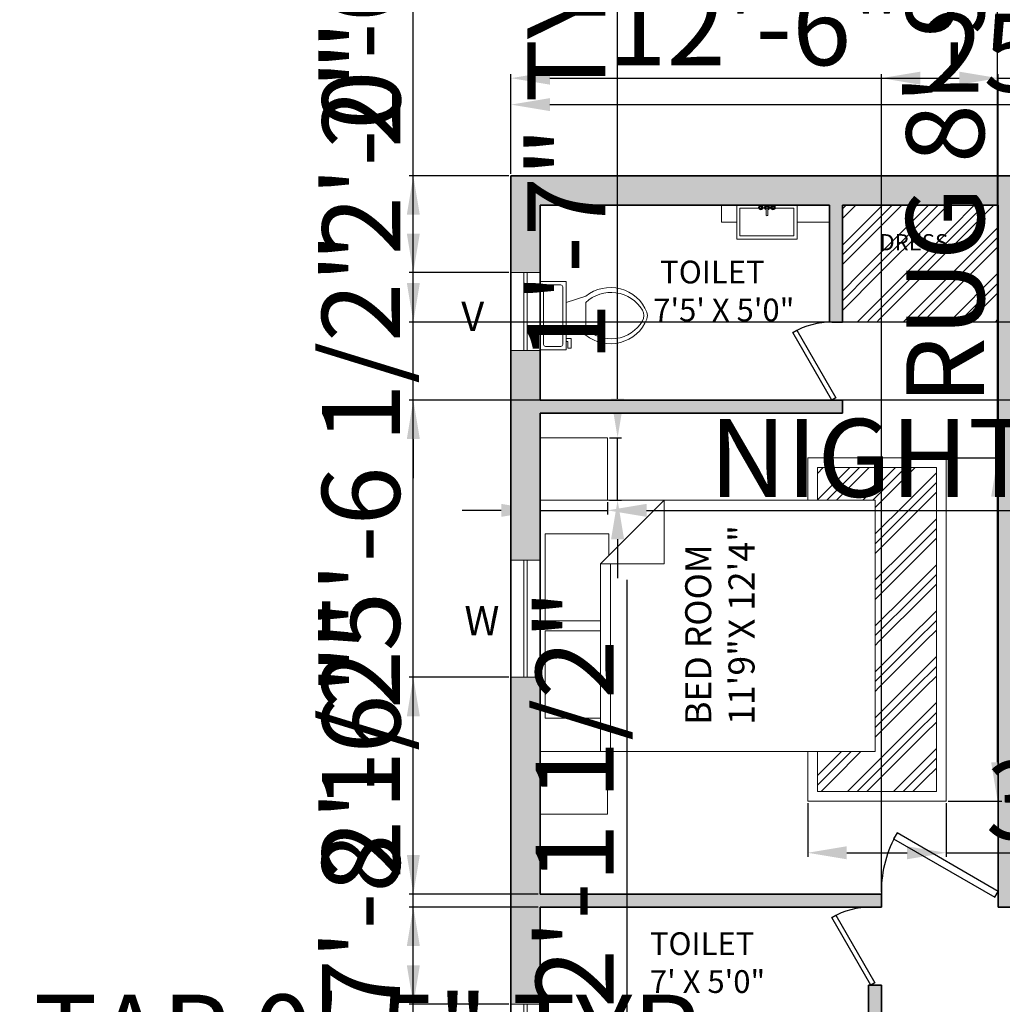
# Model space of a CAD drawing. Units: inches. Extents: x 830 to 1639, y 2591 to 3595.
# Tile 3 of 7: x 830 to 1133, y 2957 to 3260. Entities that reach past the tile are written whole.
import ezdxf

# ---------------------------------------------------------------- set-up
doc = ezdxf.new("R2010")
doc.units = ezdxf.units.IN
doc.layers.get('0').update_dxf_attribs({"color": 250})
for name, color, linetype, lineweight in [('A-ANNO-DIMS', 2, 'Continuous', 18), ('A-ANNO-TEXT', 7, 'Continuous', 18), ('A-AREA-IDEN', 7, 'Continuous', 25), ('A-DOOR', 3, 'Continuous', 25), ('A-FLOR-CASE', 8, 'Continuous', 18), ('A-FLOR-FIXT', 8, 'Continuous', 18), ('A-FLOR-PATT', 252, 'Continuous', 13), ('A-FURN', 8, 'Continuous', 18), ('A-GLAZ', 4, 'Continuous', 18), ('A-WALL', 7, 'Continuous', 35), ('A-WALL-PATT', 5, 'Continuous', 13), ('C-PROP', 7, 'Continuous', 35)]:
    doc.layers.add(name, color=color, linetype=linetype, lineweight=lineweight)
doc.styles.get("Standard").update_dxf_attribs({"font": 'arial.ttf'})
doc.dimstyles.new('ISO-25', dxfattribs={"dimtxt": 24, "dimasz": 12, "dimexe": 1.25, "dimexo": 0.625, "dimtad": 1, "dimdec": 0, "dimlunit": 3, "dimtxsty": 'Standard', "dimcen": 2.5, "dimadec": 0, "dimazin": 0, "dimtfac": 1, "dimtdec": 0, "dimtmove": 0, "dimatfit": 3, "dimfxl": 1, "dimarcsym": 0})

# ---------------------------------------------------------------- blocks, each defined once
blk = doc.blocks.new('Faucet - Bathroom top')
for p, q in [((-4.107, 0.125), (-4.375, 0.125)), ((-3.75, 0.4788), (-3.75, 0.75)), ((-3.5, 0.482), (-3.5, 0.75)), ((-3.1461, 0.125), (-2.875, 0.125)), ((3.143, 0.125), (2.875, 0.125)), ((3.5, 0.4788), (3.5, 0.75)), ((3.75, 0.482), (3.75, 0.75)), ((4.1039, 0.125), (4.375, 0.125)), ((-4.1039, -0.125), (-4.375, -0.125)), ((-3.75, -0.4821), (-3.75, -0.75)), ((-3.5, -0.4789), (-3.5, -0.75)), ((-3.143, -0.125), (-2.875, -0.125)), ((-0.5, -0.8639), (-0.5, -4.5)), ((0.5, -4.5), (0.5, -0.8631)), ((3.1461, -0.125), (2.875, -0.125)), ((3.5, -0.4821), (3.5, -0.75)), ((3.75, -0.4789), (3.75, -0.75)), ((4.107, -0.125), (4.375, -0.125))]:
    blk.add_line(p, q)
for centre, radius in [((-3.625, 0), 1.375), ((-4.625, 0), 0.2795), ((-3.625, 0), 0.5), ((-3.625, 1), 0.2795), ((-2.625, 0), 0.2795), ((0, 0), 0.5), ((3.625, 0), 1.375), ((2.625, 0), 0.2795), ((3.625, 0), 0.5), ((3.625, 1), 0.2795), ((4.625, 0), 0.2795), ((-3.625, -1), 0.2795), ((3.625, -1), 0.2795)]:
    blk.add_circle(centre, radius)
for centre, radius, start, end in [((-3.625, 0), 1, 105.2407, 164.2093), ((-3.625, 0), 1, 16.44125, 74.07887), ((0, 0), 1.5, 289.6514, 250.3603), ((0, 0), 1, 300.3431, 239.7554), ((3.625, 0), 1, 106.12, 164.0884), ((3.625, 0), 1, 16.23422, 73.90469), ((-3.625, 0), 1, 196.2342, 253.9047), ((-3.625, 0), 1, 286.12, 344.0884), ((0, -4.5), 0.5, 180, 0), ((3.625, 0), 1, 196.4413, 254.0789), ((3.625, 0), 1, 285.2407, 344.2093)]:
    blk.add_arc(centre, radius, start, end)
blk = doc.blocks.new('Bed - Queen')
for p, q in [((0, -80.00003), (0, 0)), ((0, 0), (59.99999, 0)), ((59.99999, 0), (59.99999, -80.00003)), ((7.99999, -1.2), (28.79998, -1.2)), ((7.99999, -14.4), (7.99999, -1.2)), ((28.79998, -1.2), (28.79998, -14.4)), ((31.19999, -1.2), (51.99999, -1.2)), ((31.19999, -14.4), (31.19999, -1.2)), ((51.99999, -1.2), (51.99999, -16.4)), ((0, -14.4), (44.8, -14.4)), ((59.99999, -29.6), (44.8, -14.4)), ((44.8, -14.4), (44.8, -29.6)), ((51.99999, -16.4), (46.79936, -16.4)), ((44.8, -16.8), (0, -16.8)), ((44.8, -29.6), (59.99999, -29.6)), ((59.99999, -80.00003), (0, -80.00003))]:
    blk.add_line(p, q)
blk = doc.blocks.new('Toilet - top')
for p, q in [((9.5, -6), (9.5, -2)), ((-10, -8.5), (-8, -8.5)), ((-10, -9.5), (-10, -8.5)), ((-8, -8.5), (-8, -8)), ((-7, -8), (-7, -9.5)), ((-4, -8), (-6, -14)), ((4, -8), (6, -14)), ((-7, -9.5), (-10, -9.5)), ((4, -14), (-4, -14))]:
    blk.add_line(p, q)
blk.add_lwpolyline([(10.5, -8), (10.5, 0), (-10.5, 0), (-10.5, -8)], close=True)
for points in [[(-9.5, -2), (-9.5, -6)], [(8.5, -1), (-8.5, -1)], [(-8.5, -7), (8.5, -7)]]:
    blk.add_lwpolyline(points)
for centre, radius, start, end in [((-8.62, -1.88), 0.884, 81.8699, 188.1301), ((8.62, -1.88), 0.884, 351.8699, 98.1301), ((-8.62, -6.12), 0.884, 171.8699, 278.1301), ((8.62, -6.12), 0.884, 261.8699, 8.1301), ((3.52, -21.58), 12.17, 141.4691, 247.9714), ((4.2, -21.82), 11.33, 136.3677, 238.9468), ((-3.52, -21.58), 12.17, 292.0284, 38.5307), ((-4.2, -21.82), 11.33, 301.053, 43.6321), ((0, -27.88), 4, 245.7318, 294.2682), ((0, -29), 4, 254.8605, 285.1395)]:
    blk.add_arc(centre, radius, start, end)
blk = doc.blocks.new('*U10')
for p, q in [((0, 0), (0, 100)), ((750, 0), (750, 100))]:
    blk.add_line(p, q)
blk.add_lwpolyline([(0, 0), (649.5, -375), (671.4, -337.1), (21.9, 37.9)], close=True)
blk.add_arc((0, 0), 750, 330, 0)
blk = doc.blocks.new('*U13')
for p, q in [((-750, 0), (-750, 100)), ((0, 0), (0, 100))]:
    blk.add_line(p, q)
blk.add_lwpolyline([(0, 0), (-649.5, -375), (-671.4, -337.1), (-21.9, 37.9)], close=True)
blk.add_arc((0, 0), 750, 180, 210)
blk = doc.blocks.new('*D15')
at = {"layer": 'A-ANNO-DIMS', "color": 0, "lineweight": -2, "transparency": 16777216}
for p, q in [((981.59, 3212.71), (981.59, 3235.25)), ((993.59, 3234), (1269.59, 3234)), ((1281.59, 3212.71), (1281.59, 3235.25))]:
    blk.add_line(p, q, dxfattribs=at)
at = {"layer": 'A-ANNO-DIMS', "color": 0, "transparency": 16777216}
for points in [[(993.59, 3236), (993.59, 3232), (981.59, 3234)], [(1269.59, 3236), (1269.59, 3232), (1281.59, 3234)]]:
    blk.add_solid(points, dxfattribs=at)
at = {"layer": 'Defpoints', "color": 0, "transparency": 16777216}
for p in [(1281.59, 3234), (981.59, 3212.09), (1281.59, 3212.09)]:
    blk.add_point(p, dxfattribs=at)
at = {"layer": 'A-ANNO-DIMS', "color": 0, "transparency": 16777216, "insert": (1131.59, 3246.88), "char_height": 24, "attachment_point": 5}
blk.add_mtext("25'", dxfattribs=at)
blk = doc.blocks.new('WIN-36IN')
for p, q in [((0, 0), (0, 36)), ((0, 36), (9, 36)), ((4, 0), (4, 36)), ((5, 36), (5, 0)), ((9, 36), (9, 0)), ((9, 0), (0, 0))]:
    blk.add_line(p, q)
blk = doc.blocks.new('VENT-24IN')
for p, q in [((0, 24), (9, 24)), ((0, 0), (0, 24)), ((4, 0), (4, 24)), ((5, 24), (5, 0)), ((9, 24), (9, 0)), ((9, 0), (0, 0))]:
    blk.add_line(p, q)
blk = doc.blocks.new('BEDSIDE-TABLE')
blk.add_lwpolyline([(20.72, 0), (0, 0), (0, 19.25), (20.72, 19.25)], close=True)
blk = doc.blocks.new('LAVATORY-RECT')
for points in [[(0, 10.45), (18.57, 10.45), (18.57, 0), (0, 0)], [(1, 9.45), (17.57, 9.45), (17.57, 1), (1, 1)]]:
    blk.add_lwpolyline(points, close=True)
blk = doc.blocks.new('BED-RUG-PLAN')
for points in [[(0, 92.63), (0, 105.69), (42.59, 105.69), (42.59, 0), (0, 0), (0, 15.31)], [(3, 92.63), (3, 102.69), (39.59, 102.69), (39.59, 3), (3, 3), (3, 15.31)]]:
    blk.add_lwpolyline(points)
blk = doc.blocks.new('*D26')
at = {"layer": 'A-ANNO-DIMS', "color": 0, "lineweight": -2, "transparency": 16777216}
for p, q in [((990.59, 3111.63), (990.59, 3107.9)), ((1011.31, 3111.63), (1011.31, 3107.9)), ((978.59, 3109.15), (966.59, 3109.15)), ((990.59, 3109.15), (1011.31, 3109.15)), ((1023.31, 3109.15), (1464.86, 3109.15))]:
    blk.add_line(p, q, dxfattribs=at)
at = {"layer": 'A-ANNO-DIMS', "color": 0, "transparency": 16777216}
for points in [[(978.59, 3111.15), (978.59, 3107.15), (990.59, 3109.15)], [(1023.31, 3111.15), (1023.31, 3107.15), (1011.31, 3109.15)]]:
    blk.add_solid(points, dxfattribs=at)
at = {"layer": 'Defpoints', "color": 0, "transparency": 16777216}
for p in [(990.59, 3112.26), (1011.31, 3112.26), (1011.31, 3109.15)]:
    blk.add_point(p, dxfattribs=at)
at = {"layer": 'A-ANNO-DIMS', "color": 0, "transparency": 16777216, "insert": (1250.08, 3122.18), "char_height": 24, "attachment_point": 5}
blk.add_mtext('NIGHTSTAND 1\'-8 1/2" TYP.', dxfattribs=at)
blk = doc.blocks.new('*D27')
at = {"layer": 'A-ANNO-DIMS', "color": 0, "lineweight": -2, "transparency": 16777216}
for p, q in [((1014.41, 3143.5), (1014.41, 3300.79)), ((1011.93, 3131.5), (1015.66, 3131.5)), ((1014.41, 3112.26), (1014.41, 3131.5)), ((1011.93, 3112.26), (1015.66, 3112.26)), ((1014.41, 3100.26), (1014.41, 3088.26))]:
    blk.add_line(p, q, dxfattribs=at)
at = {"layer": 'A-ANNO-DIMS', "color": 0, "transparency": 16777216}
for points in [[(1012.41, 3143.5), (1016.41, 3143.5), (1014.41, 3131.5)], [(1012.41, 3100.26), (1016.41, 3100.26), (1014.41, 3112.26)]]:
    blk.add_solid(points, dxfattribs=at)
at = {"layer": 'Defpoints', "color": 0, "transparency": 16777216}
for p in [(1011.31, 3131.5), (1014.41, 3131.5), (1011.31, 3112.26)]:
    blk.add_point(p, dxfattribs=at)
at = {"layer": 'A-ANNO-DIMS', "color": 0, "transparency": 16777216, "insert": (1001.73, 3228.15), "char_height": 24, "attachment_point": 5, "rotation": 90}
blk.add_mtext('1\'-7" TYP.', dxfattribs=at)
blk = doc.blocks.new('*D32')
at = {"layer": 'A-ANNO-DIMS', "color": 0, "lineweight": -2, "transparency": 16777216}
for p, q in [((1077.06, 2932), (1077.06, 2933.4)), ((1082.22, 2932), (1082.22, 2933.4)), ((1065.06, 2932.15), (830.39, 2932.15)), ((1082.22, 2932.15), (1077.06, 2932.15)), ((1094.22, 2932.15), (1106.22, 2932.15))]:
    blk.add_line(p, q, dxfattribs=at)
at = {"layer": 'A-ANNO-DIMS', "color": 0, "transparency": 16777216}
for points in [[(1065.06, 2934.15), (1065.06, 2930.15), (1077.06, 2932.15)], [(1094.22, 2934.15), (1094.22, 2930.15), (1082.22, 2932.15)]]:
    blk.add_solid(points, dxfattribs=at)
at = {"layer": 'Defpoints', "color": 0, "transparency": 16777216}
for p in [(1077.06, 2932.15), (1077.06, 2931.38), (1082.22, 2931.38)]:
    blk.add_point(p, dxfattribs=at)
at = {"layer": 'A-ANNO-DIMS', "color": 0, "transparency": 16777216, "insert": (941.72, 2945.03), "char_height": 24, "attachment_point": 5}
blk.add_mtext('TAP 0\'-5" TYP.', dxfattribs=at)
blk = doc.blocks.new('*D35')
at = {"layer": 'A-ANNO-DIMS', "color": 0, "lineweight": -2, "transparency": 16777216}
for p, q in [((1199.11, 3215.07), (1199.11, 3449.18)), ((1201.27, 3203.07), (1197.86, 3203.07)), ((1199.11, 3192.62), (1199.11, 3203.07)), ((1201.27, 3192.62), (1197.86, 3192.62)), ((1199.11, 3180.62), (1199.11, 3168.62))]:
    blk.add_line(p, q, dxfattribs=at)
at = {"layer": 'A-ANNO-DIMS', "color": 0, "transparency": 16777216}
for points in [[(1197.11, 3215.07), (1201.11, 3215.07), (1199.11, 3203.07)], [(1197.11, 3180.62), (1201.11, 3180.62), (1199.11, 3192.62)]]:
    blk.add_solid(points, dxfattribs=at)
at = {"layer": 'Defpoints', "color": 0, "transparency": 16777216}
for p in [(1199.11, 3203.07), (1201.9, 3203.07), (1201.9, 3192.62)]:
    blk.add_point(p, dxfattribs=at)
at = {"layer": 'A-ANNO-DIMS', "color": 0, "transparency": 16777216, "insert": (1186.08, 3338.12), "char_height": 24, "attachment_point": 5, "rotation": 90}
blk.add_mtext('0\'-10 1/2" TYP.', dxfattribs=at)
blk = doc.blocks.new('*D40')
at = {"layer": 'A-ANNO-DIMS', "color": 0, "lineweight": -2, "transparency": 16777216}
for p, q in [((1131.38, 3125.32), (1131.38, 3423.36)), ((1116.15, 3125.32), (1132.63, 3125.32)), ((1131.38, 3031.63), (1131.38, 3113.32)), ((1116.15, 3019.63), (1132.63, 3019.63))]:
    blk.add_line(p, q, dxfattribs=at)
at = {"layer": 'A-ANNO-DIMS', "color": 0, "transparency": 16777216}
for points in [[(1129.38, 3113.32), (1133.38, 3113.32), (1131.38, 3125.32)], [(1129.38, 3031.63), (1133.38, 3031.63), (1131.38, 3019.63)]]:
    blk.add_solid(points, dxfattribs=at)
at = {"layer": 'Defpoints', "color": 0, "transparency": 16777216}
for p in [(1115.52, 3125.32), (1131.38, 3125.32), (1115.52, 3019.63)]:
    blk.add_point(p, dxfattribs=at)
at = {"layer": 'A-ANNO-DIMS', "color": 0, "transparency": 16777216, "insert": (1118.34, 3280.34), "char_height": 24, "attachment_point": 5, "rotation": 90}
blk.add_mtext('RUG 8\'-9 1/2" TYP.', dxfattribs=at)
blk = doc.blocks.new('*D41')
at = {"layer": 'A-ANNO-DIMS', "color": 0, "lineweight": -2, "transparency": 16777216}
for p, q in [((1072.93, 3019), (1072.93, 3002.53)), ((1115.52, 3019), (1115.52, 3002.53)), ((1084.93, 3003.78), (1103.52, 3003.78)), ((1115.52, 3003.78), (1330.97, 3003.78))]:
    blk.add_line(p, q, dxfattribs=at)
at = {"layer": 'A-ANNO-DIMS', "color": 0, "transparency": 16777216}
for points in [[(1084.93, 3005.78), (1084.93, 3001.78), (1072.93, 3003.78)], [(1103.52, 3005.78), (1103.52, 3001.78), (1115.52, 3003.78)]]:
    blk.add_solid(points, dxfattribs=at)
at = {"layer": 'Defpoints', "color": 0, "transparency": 16777216}
for p in [(1072.93, 3019.63), (1115.52, 3019.63), (1115.52, 3003.78)]:
    blk.add_point(p, dxfattribs=at)
at = {"layer": 'A-ANNO-DIMS', "color": 0, "transparency": 16777216, "insert": (1229.25, 3016.82), "char_height": 24, "attachment_point": 5}
blk.add_mtext('3\'-6 1/2" TYP.', dxfattribs=at)
blk = doc.blocks.new('*D44')
at = {"layer": 'A-ANNO-DIMS', "color": 0, "lineweight": -2, "transparency": 16777216}
for p, q in [((1017.38, 2827.49), (1017.38, 3087.77)), ((1014.18, 2827.49), (1018.63, 2827.49)), ((1017.38, 2814.04), (1017.38, 2815.49)), ((1014.18, 2802.04), (1018.63, 2802.04))]:
    blk.add_line(p, q, dxfattribs=at)
at = {"layer": 'A-ANNO-DIMS', "color": 0, "transparency": 16777216}
for points in [[(1015.38, 2815.49), (1019.38, 2815.49), (1017.38, 2827.49)], [(1015.38, 2814.04), (1019.38, 2814.04), (1017.38, 2802.04)]]:
    blk.add_solid(points, dxfattribs=at)
at = {"layer": 'Defpoints', "color": 0, "transparency": 16777216}
for p in [(1013.56, 2827.49), (1017.38, 2827.49), (1013.56, 2802.04)]:
    blk.add_point(p, dxfattribs=at)
at = {"layer": 'A-ANNO-DIMS', "color": 0, "transparency": 16777216, "insert": (1004.34, 2963.63), "char_height": 24, "attachment_point": 5, "rotation": 90}
blk.add_mtext('RANGE 2\'-1 1/2"', dxfattribs=at)
blk = doc.blocks.new('*D49')
at = {"layer": 'A-ANNO-DIMS', "color": 0, "lineweight": -2, "transparency": 16777216}
for p, q in [((1095.59, 2991.71), (1095.59, 3243.39)), ((1107.59, 3242.14), (1119.59, 3242.14)), ((1131.59, 2992.51), (1131.59, 3243.39)), ((1131.59, 3242.14), (1208.62, 3242.14))]:
    blk.add_line(p, q, dxfattribs=at)
at = {"layer": 'A-ANNO-DIMS', "color": 0, "transparency": 16777216}
for points in [[(1107.59, 3244.14), (1107.59, 3240.14), (1095.59, 3242.14)], [(1119.59, 3244.14), (1119.59, 3240.14), (1131.59, 3242.14)]]:
    blk.add_solid(points, dxfattribs=at)
at = {"layer": 'Defpoints', "color": 0, "transparency": 16777216}
for p in [(1131.59, 3242.14), (1095.59, 2991.09), (1131.59, 2991.89)]:
    blk.add_point(p, dxfattribs=at)
at = {"layer": 'A-ANNO-DIMS', "color": 0, "transparency": 16777216, "insert": (1176.11, 3255.02), "char_height": 24, "attachment_point": 5}
blk.add_mtext('3\'-0"', dxfattribs=at)
blk = doc.blocks.new('*D50')
at = {"layer": 'A-ANNO-DIMS', "color": 0, "lineweight": -2, "transparency": 16777216}
for p, q in [((951.54, 3179.09), (951.54, 3256.54)), ((1187.96, 3167.09), (950.29, 3167.09)), ((951.54, 3143.09), (951.54, 3167.09)), ((1187.96, 3143.09), (950.29, 3143.09)), ((951.54, 3131.09), (951.54, 3119.09))]:
    blk.add_line(p, q, dxfattribs=at)
at = {"layer": 'A-ANNO-DIMS', "color": 0, "transparency": 16777216}
for points in [[(949.54, 3179.09), (953.54, 3179.09), (951.54, 3167.09)], [(949.54, 3131.09), (953.54, 3131.09), (951.54, 3143.09)]]:
    blk.add_solid(points, dxfattribs=at)
at = {"layer": 'Defpoints', "color": 0, "transparency": 16777216}
for p in [(951.54, 3167.09), (1188.59, 3167.09), (1188.59, 3143.09)]:
    blk.add_point(p, dxfattribs=at)
at = {"layer": 'A-ANNO-DIMS', "color": 0, "transparency": 16777216, "insert": (938.66, 3223.82), "char_height": 24, "attachment_point": 5, "rotation": 90}
blk.add_mtext('2\'-0"', dxfattribs=at)
blk = doc.blocks.new('*D57')
at = {"layer": 'A-ANNO-DIMS', "color": 0, "lineweight": -2, "transparency": 16777216}
for p, q in [((951.54, 2944.9), (951.54, 3077.67)), ((1203.59, 2944.9), (950.29, 2944.9)), ((951.54, 2864.53), (951.54, 2932.9)), ((1203.59, 2852.53), (950.29, 2852.53))]:
    blk.add_line(p, q, dxfattribs=at)
at = {"layer": 'A-ANNO-DIMS', "color": 0, "transparency": 16777216}
for points in [[(949.54, 2932.9), (953.54, 2932.9), (951.54, 2944.9)], [(949.54, 2864.53), (953.54, 2864.53), (951.54, 2852.53)]]:
    blk.add_solid(points, dxfattribs=at)
at = {"layer": 'Defpoints', "color": 0, "transparency": 16777216}
for p in [(951.54, 2944.9), (1204.22, 2944.9), (1204.22, 2852.53)]:
    blk.add_point(p, dxfattribs=at)
at = {"layer": 'A-ANNO-DIMS', "color": 0, "transparency": 16777216, "insert": (938.51, 3017.28), "char_height": 24, "attachment_point": 5, "rotation": 90}
blk.add_mtext('7\'-8 1/2"', dxfattribs=at)
blk = doc.blocks.new('*D58')
at = {"layer": 'A-ANNO-DIMS', "color": 0, "lineweight": -2, "transparency": 16777216}
for p, q in [((981.59, 3212.71), (981.59, 3243.39)), ((993.59, 3242.14), (1119.59, 3242.14)), ((1131.59, 3203.71), (1131.59, 3243.39))]:
    blk.add_line(p, q, dxfattribs=at)
at = {"layer": 'A-ANNO-DIMS', "color": 0, "transparency": 16777216}
for points in [[(993.59, 3244.14), (993.59, 3240.14), (981.59, 3242.14)], [(1119.59, 3244.14), (1119.59, 3240.14), (1131.59, 3242.14)]]:
    blk.add_solid(points, dxfattribs=at)
at = {"layer": 'Defpoints', "color": 0, "transparency": 16777216}
for p in [(1131.59, 3242.14), (981.59, 3212.09), (1131.59, 3203.09)]:
    blk.add_point(p, dxfattribs=at)
at = {"layer": 'A-ANNO-DIMS', "color": 0, "transparency": 16777216, "insert": (1056.59, 3255.02), "char_height": 24, "attachment_point": 5}
blk.add_mtext('12\'-6"', dxfattribs=at)
blk = doc.blocks.new('*D61')
at = {"layer": 'A-ANNO-DIMS', "color": 0, "lineweight": -2, "transparency": 16777216}
for p, q in [((951.54, 3057.79), (951.54, 3190.76)), ((980.96, 3057.79), (950.29, 3057.79)), ((951.54, 3003.09), (951.54, 3045.79)), ((989.96, 2991.09), (950.29, 2991.09))]:
    blk.add_line(p, q, dxfattribs=at)
at = {"layer": 'A-ANNO-DIMS', "color": 0, "transparency": 16777216}
for points in [[(949.54, 3045.79), (953.54, 3045.79), (951.54, 3057.79)], [(949.54, 3003.09), (953.54, 3003.09), (951.54, 2991.09)]]:
    blk.add_solid(points, dxfattribs=at)
at = {"layer": 'Defpoints', "color": 0, "transparency": 16777216}
for p in [(951.54, 3057.79), (981.59, 3057.79), (990.59, 2991.09)]:
    blk.add_point(p, dxfattribs=at)
at = {"layer": 'A-ANNO-DIMS', "color": 0, "transparency": 16777216, "insert": (938.51, 3130.27), "char_height": 24, "attachment_point": 5, "rotation": 90}
blk.add_mtext('5\'-6 1/2"', dxfattribs=at)
blk = doc.blocks.new('*D69')
at = {"layer": 'A-ANNO-DIMS', "color": 0, "lineweight": -2, "transparency": 16777216}
for p, q in [((951.54, 3212.09), (951.54, 3289.54)), ((980.96, 3212.09), (950.29, 3212.09)), ((951.54, 3194.32), (951.54, 3200.09)), ((980.96, 3182.32), (950.29, 3182.32))]:
    blk.add_line(p, q, dxfattribs=at)
at = {"layer": 'A-ANNO-DIMS', "color": 0, "transparency": 16777216}
for points in [[(949.54, 3200.09), (953.54, 3200.09), (951.54, 3212.09)], [(949.54, 3194.32), (953.54, 3194.32), (951.54, 3182.32)]]:
    blk.add_solid(points, dxfattribs=at)
at = {"layer": 'Defpoints', "color": 0, "transparency": 16777216}
for p in [(951.54, 3212.09), (981.59, 3212.09), (981.59, 3182.32)]:
    blk.add_point(p, dxfattribs=at)
at = {"layer": 'A-ANNO-DIMS', "color": 0, "transparency": 16777216, "insert": (938.66, 3256.82), "char_height": 24, "attachment_point": 5, "rotation": 90}
blk.add_mtext('2\'-6"', dxfattribs=at)
blk = doc.blocks.new('*D71')
at = {"layer": 'A-ANNO-DIMS', "color": 0, "lineweight": -2, "transparency": 16777216}
for p, q in [((951.54, 2987.09), (951.54, 3064.54)), ((989.96, 2987.09), (950.29, 2987.09)), ((951.54, 2969.15), (951.54, 2975.09)), ((980.96, 2957.15), (950.29, 2957.15))]:
    blk.add_line(p, q, dxfattribs=at)
at = {"layer": 'A-ANNO-DIMS', "color": 0, "transparency": 16777216}
for points in [[(949.54, 2975.09), (953.54, 2975.09), (951.54, 2987.09)], [(949.54, 2969.15), (953.54, 2969.15), (951.54, 2957.15)]]:
    blk.add_solid(points, dxfattribs=at)
at = {"layer": 'Defpoints', "color": 0, "transparency": 16777216}
for p in [(951.54, 2987.09), (990.59, 2987.09), (981.59, 2957.15)]:
    blk.add_point(p, dxfattribs=at)
at = {"layer": 'A-ANNO-DIMS', "color": 0, "transparency": 16777216, "insert": (938.66, 3031.82), "char_height": 24, "attachment_point": 5, "rotation": 90}
blk.add_mtext('2\'-6"', dxfattribs=at)

msp = doc.modelspace()

# ---------------------------------------------------------------- hatches: boundary and pattern name
at = {"layer": 'A-FLOR-PATT'}
h = msp.add_hatch(dxfattribs=at)
h.set_pattern_fill('GOST_GROUND', color=256)
h.paths.add_polyline_path([(1112.52, 3122.32), (1075.93, 3122.32), (1075.93, 3112.26), (1093.69, 3112.26), (1093.69, 3034.94), (1075.93, 3034.94), (1075.93, 3022.63), (1112.52, 3022.63)])
h.paths.add_polyline_path([(1169.49, 3115.15), (1187.25, 3115.15), (1187.25, 3127.45), (1150.65, 3127.45), (1150.65, 3027.77), (1187.25, 3027.77), (1187.25, 3037.83), (1169.49, 3037.83)])
h.paths.add_polyline_path([(1131.59, 3203.09), (1083.59, 3203.09), (1083.59, 3167.09), (1131.59, 3167.09)])
h.paths.add_polyline_path([(1188.59, 3203.09), (1140.59, 3203.09), (1140.59, 3167.09), (1188.59, 3167.09)])
at = {"layer": 'A-WALL-PATT'}
h = msp.add_hatch(color=256, dxfattribs=at)
h.dxf.hatch_style = 1
h.paths.add_polyline_path([(990.59, 3203.09), (1079.59, 3203.09), (1079.59, 3167.09), (1083.59, 3167.09), (1083.59, 3203.09), (1131.59, 3203.09), (1131.59, 2987.09), (1140.59, 2987.09), (1140.59, 2991.89), (1140.59, 3203.09), (1188.59, 3203.09), (1188.59, 3167.09), (1192.59, 3167.09), (1192.59, 3203.09), (1272.59, 3203.09), (1272.59, 3181.45), (1281.59, 3181.45), (1281.59, 3212.09), (981.59, 3212.09), (981.59, 3182.32), (990.59, 3182.32)])
h = msp.add_hatch(color=256, dxfattribs=at)
h.dxf.hatch_style = 1
h.paths.add_polyline_path([(981.59, 3093.79), (990.59, 3093.79), (990.59, 3112.26), (990.59, 3131.5), (990.59, 3139.09), (1083.59, 3139.09), (1083.59, 3143.09), (1080.39, 3143.09), (990.59, 3143.09), (990.59, 3158.32), (981.59, 3158.32)])
h = msp.add_hatch(color=256, dxfattribs=at)
h.dxf.hatch_style = 1
h.paths.add_polyline_path([(981.59, 2957.15), (990.59, 2957.15), (990.59, 2987.09), (1095.59, 2987.09), (1095.59, 2991.09), (990.59, 2991.09), (990.59, 3057.79), (981.59, 3057.79)])
h = msp.add_hatch(color=256, dxfattribs=at)
h.dxf.hatch_style = 1
h.paths.add_polyline_path([(1091.59, 2923.09), (1091.59, 2859.09), (1095.59, 2859.09), (1095.59, 2963.09), (1091.59, 2963.09), (1091.59, 2927.09), (990.59, 2927.09), (990.59, 2923.09)])

# ---------------------------------------------------------------- linework, layer by layer
at = {"layer": 'A-FLOR-CASE'}
for p, q in [((1046.39, 3197.86), (1046.39, 3203.09)), ((1051.08, 3197.86), (1046.39, 3197.86)), ((1069.64, 3197.86), (1079.59, 3197.86)), ((1079.59, 3167.09), (1131.59, 3167.09))]:
    msp.add_line(p, q, dxfattribs=at)
at = {"layer": 'A-WALL'}
for p, q in [((990.59, 3203.09), (1079.59, 3203.09)), ((990.59, 3143.09), (990.59, 3203.09)), ((1079.59, 3167.09), (1079.59, 3203.09)), ((1083.59, 3167.09), (1083.59, 3203.09)), ((1083.59, 3203.09), (1131.59, 3203.09)), ((1131.59, 2987.09), (1131.59, 3203.09)), ((990.59, 3143.09), (1083.59, 3143.09)), ((1083.59, 3139.09), (1083.59, 3143.09)), ((990.59, 3139.09), (1083.59, 3139.09)), ((990.59, 2991.09), (990.59, 3139.09)), ((1095.59, 2987.09), (1095.59, 2991.09)), ((990.59, 2863.09), (990.59, 2987.09)), ((1091.59, 2927.09), (1091.59, 2963.09)), ((1095.59, 2859.09), (1095.59, 2963.09))]:
    msp.add_line(p, q, dxfattribs=at)
for points in [[(990.59, 2991.09), (1095.59, 2991.09)], [(990.59, 2987.09), (1095.59, 2987.09)], [(1131.59, 2987.09), (1140.59, 2987.09)], [(1091.59, 2963.09), (1095.59, 2963.09)]]:
    msp.add_lwpolyline(points, dxfattribs=at)
at = {"layer": 'C-PROP'}
msp.add_lwpolyline([(981.59, 3212.09), (1281.59, 3212.09), (1281.59, 2672.09), (981.59, 2672.09)], close=True, dxfattribs=at)

# ---------------------------------------------------------------- block references
at = {"layer": 'A-DOOR'}
for name, p, xscale, yscale, zscale, rotation in [('*U13', (1080.39, 3143.09), 0.032, 0.032, 0.032, 270), ('*U10', (1131.59, 2991.89), 0.0480000000000001, 0.0480000000000001, 0.0480000000000001, 180), ('*U13', (1092.39, 2963.09), 0.032, 0.032, 0.032, 270)]:
    msp.add_blockref(name, p, dxfattribs=dict(at, xscale=xscale, yscale=yscale, zscale=zscale, rotation=rotation))
at = {"layer": 'A-FLOR-FIXT'}
msp.add_blockref('LAVATORY-RECT', (1051.08, 3192.64), dxfattribs=at)
at = {"layer": 'A-FLOR-FIXT', "xscale": 0.5159985736076383, "yscale": 0.5159985736076383, "zscale": 0.5159985736076383}
msp.add_blockref('Faucet - Bathroom top', (1060.36, 3202.35), dxfattribs=at)
at = {"layer": 'A-FLOR-FIXT', "rotation": 90}
msp.add_blockref('Toilet - top', (990.59, 3169.07), dxfattribs=at)
at = {"layer": 'A-FURN'}
for name, p in [('BEDSIDE-TABLE', (990.59, 3112.26)), ('BED-RUG-PLAN', (1072.93, 3019.63)), ('BEDSIDE-TABLE', (990.59, 3015.69))]:
    msp.add_blockref(name, p, dxfattribs=at)
at = {"layer": 'A-FURN', "xscale": 1.288695656948927, "yscale": 1.288695656948927, "zscale": 1.288695656948927, "rotation": 90}
msp.add_blockref('Bed - Queen', (990.59, 3034.94), dxfattribs=at)
at = {"layer": 'A-GLAZ'}
for name, p in [('VENT-24IN', (981.59, 3158.32)), ('WIN-36IN', (981.59, 3057.79)), ('VENT-24IN', (981.59, 2933.15))]:
    msp.add_blockref(name, p, dxfattribs=at)

# ---------------------------------------------------------------- texts
at = {"layer": 'A-ANNO-TEXT', "insert": (966.28, 3173.36), "char_height": 9, "attachment_point": 1}
msp.add_mtext_dynamic_manual_height_columns('{\\fArial|b1|i0|c0|p34;V}', width=72.2202, gutter_width=12.5, heights=[0], dxfattribs=at)
at = {"layer": 'A-ANNO-TEXT', "insert": (967.26, 3079.74), "char_height": 9, "width": 31.3961, "attachment_point": 1}
msp.add_mtext('{\\fArial|b1|i0|c0|p34;W}', dxfattribs=at)
at = {"layer": 'A-AREA-IDEN', "attachment_point": 1}
for s, width, heights, insert, char_height in [('{\\fArial|b1|i0|c0|p34;DRESS}', 42.669, [25.05], (1094.99, 3194.14), 5), ('{\\fArial|b1|i0|c0|p34; TOILET \\P7\'5\' X 5\'0"}', 48.1377, [35.05], (1025.38, 3185.98), 7)]:
    msp.add_mtext_dynamic_manual_height_columns(s, width=width, gutter_width=12.5, heights=heights, dxfattribs=dict(at, insert=insert, char_height=char_height))
at = {"layer": 'A-AREA-IDEN', "insert": (1035.22, 3043.16), "char_height": 8, "width": 92.8024, "attachment_point": 1, "rotation": 90}
msp.add_mtext('{\\fArial|b1|i0|c0|p34;BED ROOM\\P11\'9"X 12\'4"}', dxfattribs=at)
at = {"layer": 'A-AREA-IDEN', "insert": (1024.35, 2979.32), "char_height": 7, "width": 63.8983, "attachment_point": 1}
msp.add_mtext('{\\fArial|b1|i0|c0|p34;TOILET \\P7\' X 5\'0"}', dxfattribs=at)

# ---------------------------------------------------------------- dimensions: what is measured, and where the dimension line sits
at = {"layer": 'A-ANNO-DIMS'}
for base, p1, p2, angle, text, picture, middle in [((1199.1117, 3203.0656), (1201.8966, 3192.6174), (1201.8966, 3203.0656), 90, '<> TYP.', '*D35', (1186.0775, 3338.1217)), ((1131.38, 3125.32), (1115.52, 3019.63), (1115.52, 3125.32), 90, 'RUG <> TYP.', '*D40', (1118.34, 3280.34)), ((1014.41, 3131.5), (1011.31, 3112.26), (1011.31, 3131.5), 90, '<> TYP.', '*D27', (1001.73, 3228.15)), ((1017.3756, 2827.4932), (1013.5572, 2802.0374), (1013.5572, 2827.4932), 90, 'RANGE <>', '*D44', (1004.3413, 2963.6298)), ((1077.06, 2932.15), (1082.22, 2931.38), (1077.06, 2931.38), 180, 'TAP <> TYP.', '*D32', (941.72, 2945.03))]:
    dim = msp.add_linear_dim(base=base, p1=p1, p2=p2, angle=angle, text=text, dimstyle='ISO-25', override={"dimdec": 1, "dimlfac": 1, "dimrnd": 0, "dimzin": 1, "dimdsep": 46, "dimlunit": 4, "dimfrac": 2}, dxfattribs=at)
    dim.commit()
    dim.dimension.update_dxf_attribs({"geometry": picture, "text_midpoint": middle})
for base, p1, p2, picture, middle in [((951.54, 3212.09), (981.59, 3182.32), (981.59, 3212.09), '*D69', (938.66, 3256.82)), ((951.54, 3167.09), (1188.59, 3143.09), (1188.59, 3167.09), '*D50', (938.66, 3223.82)), ((951.54, 3057.79), (990.59, 2991.09), (981.59, 3057.79), '*D61', (938.51, 3130.27)), ((951.54, 2944.9), (1204.22, 2852.53), (1204.22, 2944.9), '*D57', (938.51, 3017.28)), ((951.54, 2987.09), (981.59, 2957.15), (990.59, 2987.09), '*D71', (938.66, 3031.82))]:
    dim = msp.add_linear_dim(base=base, p1=p1, p2=p2, angle=90, dimstyle='ISO-25', override={"dimdec": 1, "dimlfac": 1, "dimrnd": 0, "dimzin": 1, "dimdsep": 46, "dimlunit": 4, "dimfrac": 2}, dxfattribs=at)
    dim.commit()
    dim.dimension.update_dxf_attribs({"geometry": picture, "text_midpoint": middle})
for base, p1, p2, override, picture, middle in [((1131.59, 3242.14), (981.59, 3212.09), (1131.59, 3203.09), {"dimdec": 1, "dimlfac": 1, "dimrnd": 0, "dimzin": 1, "dimdsep": 46, "dimlunit": 4, "dimfrac": 2}, '*D58', (1056.59, 3255.02)), ((1131.59, 3242.14), (1095.59, 2991.09), (1131.59, 2991.89), {"dimdec": 1, "dimlfac": 1, "dimrnd": 0, "dimzin": 1, "dimdsep": 46, "dimlunit": 4, "dimfrac": 2}, '*D49', (1176.11, 3255.02)), ((1281.59, 3234), (981.59, 3212.09), (1281.59, 3212.09), {"dimclrd": 0, "dimclre": 0, "dimclrt": 0}, '*D15', (1131.59, 3246.88))]:
    dim = msp.add_linear_dim(base=base, p1=p1, p2=p2, dimstyle='ISO-25', override=override, dxfattribs=at)
    dim.commit()
    dim.dimension.update_dxf_attribs({"geometry": picture, "text_midpoint": middle})
for base, p1, p2, text, picture, middle in [((1011.31, 3109.15), (990.59, 3112.26), (1011.31, 3112.26), 'NIGHTSTAND <> TYP.', '*D26', (1250.08, 3122.18)), ((1115.52, 3003.78), (1072.93, 3019.63), (1115.52, 3019.63), '<> TYP.', '*D41', (1229.25, 3016.82))]:
    dim = msp.add_linear_dim(base=base, p1=p1, p2=p2, text=text, dimstyle='ISO-25', override={"dimdec": 1, "dimlfac": 1, "dimrnd": 0, "dimzin": 1, "dimdsep": 46, "dimlunit": 4, "dimfrac": 2}, dxfattribs=at)
    dim.commit()
    dim.dimension.update_dxf_attribs({"geometry": picture, "text_midpoint": middle})

doc.saveas('drawing.dxf')
